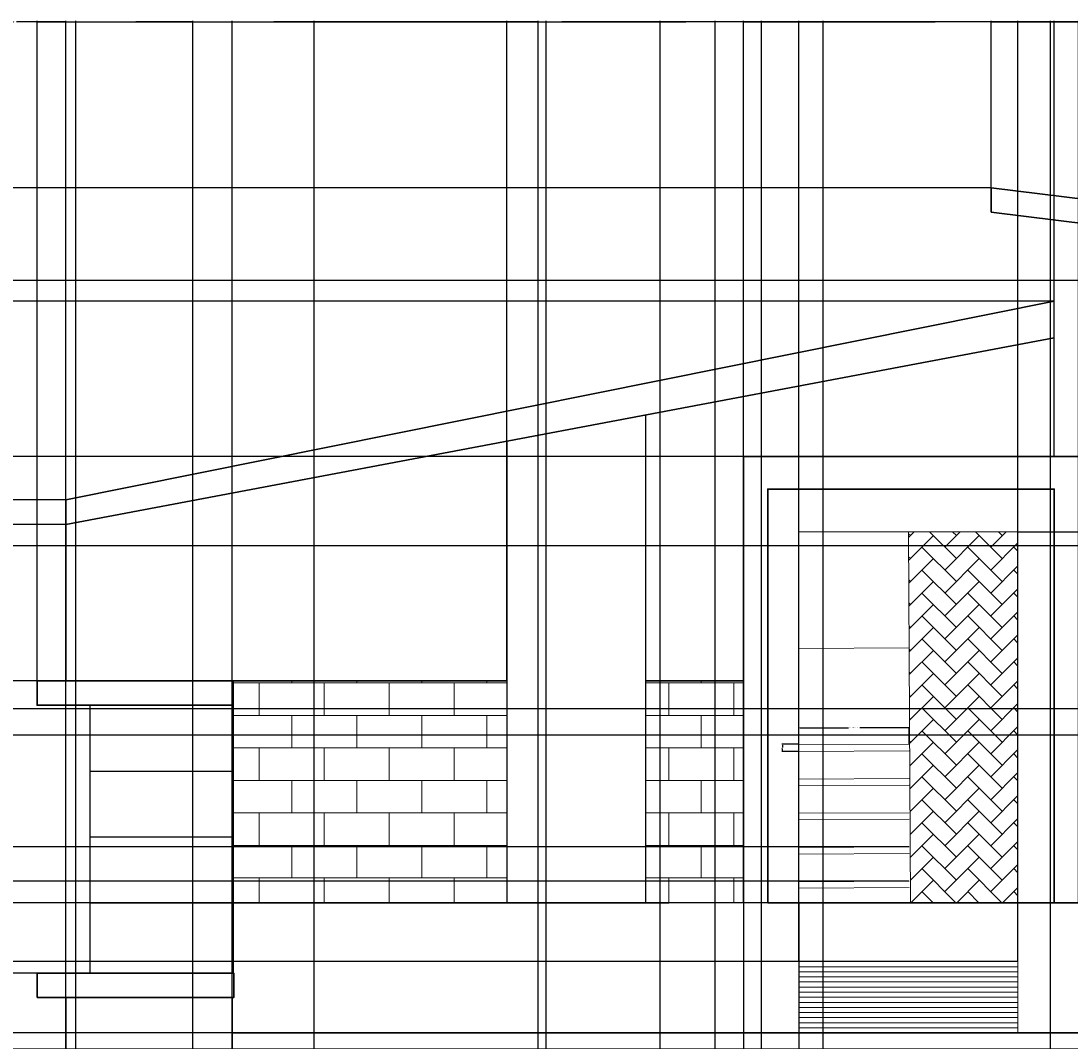
# Model space of a CAD drawing. Units: inches. Extents: x -14 to 886, y 45 to 435.
# Tile 3 of 5: x 125 to 384, y 184 to 435. Entities that reach past the tile are written whole.
import ezdxf

# ---------------------------------------------------------------- set-up
doc = ezdxf.new("R2010")
doc.units = ezdxf.units.IN
doc.header["$MEASUREMENT"] = 0
for name, color, linetype, lineweight in [('A-ANNO-DIMS', 2, 'Continuous', 18), ('A-ELEV-BAND', 7, 'Continuous', 30), ('A-ELEV-PATT', 252, 'Continuous', 13), ('A-ELEV-SCRN', 8, 'Continuous', 18), ('A-ROOF', 7, 'Continuous', 35), ('A-WALL', 7, 'Continuous', 25), ('A-WALL-PATT', 252, 'Continuous', 13), ('L-WALL', 7, 'Continuous', 30)]:
    doc.layers.add(name, color=color, linetype=linetype, lineweight=lineweight)
doc.styles.get("Standard").update_dxf_attribs({"font": 'arial.ttf'})
doc.dimstyles.get("Standard").update_dxf_attribs({"dimtxt": 0.18, "dimasz": 0.18, "dimexe": 0.18, "dimexo": 0.0625, "dimgap": 0.09, "dimtad": 0, "dimtih": 1, "dimtoh": 1, "dimdec": 4, "dimzin": 0, "dimdsep": 46, "dimtxsty": 'Standard', "dimcen": 0.09, "dimadec": 0, "dimazin": 0, "dimtfac": 1, "dimtdec": 4, "dimtofl": 0, "dimtmove": 0, "dimatfit": 3, "dimfxl": 1, "dimtolj": 1, "dimtzin": 0, "dimarcsym": 0})

# ---------------------------------------------------------------- blocks, each defined once
blk = doc.blocks.new('SCREEN-HORIZONTAL-BAR')
for p, q in [((0, 1.61), (27.14, 1.76)), ((0, 0), (27.14, 0.16))]:
    blk.add_line(p, q)
blk = doc.blocks.new('*D6')
at = {"layer": 'A-ANNO-DIMS', "color": 0, "lineweight": -2, "transparency": 16777216}
for p, q in [((316.91, 256.97), (316.91, 261.16)), ((317.09, 260.98), (329.1, 260.98)), ((343.87, 260.98), (331.86, 260.98)), ((344.05, 256.97), (344.05, 261.16))]:
    blk.add_line(p, q, dxfattribs=at)
at = {"layer": 'A-ANNO-DIMS', "color": 0, "transparency": 16777216}
for points in [[(317.09, 261.01), (317.09, 260.95), (316.91, 260.98)], [(343.87, 261.01), (343.87, 260.95), (344.05, 260.98)]]:
    blk.add_solid(points, dxfattribs=at)
at = {"layer": 'Defpoints', "color": 0, "transparency": 16777216}
for p in [(344.05, 260.98), (316.91, 256.91), (344.05, 256.91)]:
    blk.add_point(p, dxfattribs=at)
at = {"layer": 'A-ANNO-DIMS', "color": 0, "transparency": 16777216, "insert": (330.48, 260.98), "char_height": 0.18, "attachment_point": 5}
blk.add_mtext('\\A1;SCREEN BAR 27 TYP.', dxfattribs=at)
blk = doc.blocks.new('*D7')
at = {"layer": 'A-ANNO-DIMS', "color": 0, "lineweight": -2, "transparency": 16777216}
for p, q in [((316.85, 256.91), (312.66, 256.91)), ((312.84, 256.73), (312.84, 256.21)), ((316.85, 255.15), (312.66, 255.15)), ((312.84, 255.33), (312.84, 255.85))]:
    blk.add_line(p, q, dxfattribs=at)
at = {"layer": 'A-ANNO-DIMS', "color": 0, "transparency": 16777216}
for points in [[(312.81, 256.73), (312.87, 256.73), (312.84, 256.91)], [(312.81, 255.33), (312.87, 255.33), (312.84, 255.15)]]:
    blk.add_solid(points, dxfattribs=at)
at = {"layer": 'Defpoints', "color": 0, "transparency": 16777216}
for p in [(312.84, 256.91), (316.91, 256.91), (316.91, 255.15)]:
    blk.add_point(p, dxfattribs=at)
at = {"layer": 'A-ANNO-DIMS', "color": 0, "transparency": 16777216, "insert": (312.84, 256.03), "char_height": 0.18, "attachment_point": 5}
blk.add_mtext('\\A1;2 TYP.', dxfattribs=at)
blk = doc.blocks.new('*D17')
at = {"layer": 'A-ANNO-DIMS', "color": 0, "lineweight": -2, "transparency": 16777216}
for p, q in [((364.17, 393.98), (-13.96, 393.98)), ((-13.78, 393.8), (-13.78, 240.44)), ((-13.78, 86.72), (-13.78, 240.08)), ((111.24, 86.54), (-13.96, 86.54))]:
    blk.add_line(p, q, dxfattribs=at)
at = {"layer": 'A-ANNO-DIMS', "color": 0, "transparency": 16777216}
for points in [[(-13.81, 393.8), (-13.75, 393.8), (-13.78, 393.98)], [(-13.81, 86.72), (-13.75, 86.72), (-13.78, 86.54)]]:
    blk.add_solid(points, dxfattribs=at)
at = {"layer": 'Defpoints', "color": 0, "transparency": 16777216}
for p in [(-13.78, 393.98), (364.23, 393.98), (111.3, 86.54)]:
    blk.add_point(p, dxfattribs=at)
at = {"layer": 'A-ANNO-DIMS', "color": 0, "transparency": 16777216, "insert": (-13.78, 240.26), "char_height": 0.18, "attachment_point": 5}
blk.add_mtext('\\A1;307.44', dxfattribs=at)
blk = doc.blocks.new('*D24')
at = {"layer": 'A-ANNO-DIMS', "color": 0, "lineweight": -2, "transparency": 16777216}
for p, q in [((136.31, 311.03), (-13.96, 311.03)), ((-13.78, 310.85), (-13.78, 198.97)), ((-13.78, 86.72), (-13.78, 198.6)), ((195.24, 86.54), (-13.96, 86.54))]:
    blk.add_line(p, q, dxfattribs=at)
at = {"layer": 'A-ANNO-DIMS', "color": 0, "transparency": 16777216}
for points in [[(-13.81, 310.85), (-13.75, 310.85), (-13.78, 311.03)], [(-13.81, 86.72), (-13.75, 86.72), (-13.78, 86.54)]]:
    blk.add_solid(points, dxfattribs=at)
at = {"layer": 'Defpoints', "color": 0, "transparency": 16777216}
for p in [(-13.78, 311.03), (136.37, 311.03), (195.3, 86.54)]:
    blk.add_point(p, dxfattribs=at)
at = {"layer": 'A-ANNO-DIMS', "color": 0, "transparency": 16777216, "insert": (-13.78, 198.79), "char_height": 0.18, "attachment_point": 5}
blk.add_mtext('\\A1;224.5', dxfattribs=at)
blk = doc.blocks.new('*D25')
at = {"layer": 'A-ANNO-DIMS', "color": 0, "lineweight": -2, "transparency": 16777216}
for p, q in [((136.37, 317.16), (136.37, 435.05)), ((136.55, 434.87), (257.59, 434.87)), ((379.56, 434.87), (258.52, 434.87)), ((379.74, 366.09), (379.74, 435.05))]:
    blk.add_line(p, q, dxfattribs=at)
at = {"layer": 'A-ANNO-DIMS', "color": 0, "transparency": 16777216}
for points in [[(136.55, 434.9), (136.55, 434.84), (136.37, 434.87)], [(379.56, 434.9), (379.56, 434.84), (379.74, 434.87)]]:
    blk.add_solid(points, dxfattribs=at)
at = {"layer": 'Defpoints', "color": 0, "transparency": 16777216}
for p in [(379.74, 434.87), (379.74, 366.03), (136.37, 317.1)]:
    blk.add_point(p, dxfattribs=at)
at = {"layer": 'A-ANNO-DIMS', "color": 0, "transparency": 16777216, "insert": (258.05, 434.87), "char_height": 0.18, "attachment_point": 5}
blk.add_mtext('\\A1;243.36', dxfattribs=at)
blk = doc.blocks.new('*D26')
at = {"layer": 'A-ANNO-DIMS', "color": 0, "lineweight": -2, "transparency": 16777216}
for p, q in [((379.67, 366.03), (-13.96, 366.03)), ((-13.78, 365.85), (-13.78, 341.75)), ((-13.78, 317.28), (-13.78, 341.38)), ((136.31, 317.1), (-13.96, 317.1))]:
    blk.add_line(p, q, dxfattribs=at)
at = {"layer": 'A-ANNO-DIMS', "color": 0, "transparency": 16777216}
for points in [[(-13.81, 365.85), (-13.75, 365.85), (-13.78, 366.03)], [(-13.81, 317.28), (-13.75, 317.28), (-13.78, 317.1)]]:
    blk.add_solid(points, dxfattribs=at)
at = {"layer": 'Defpoints', "color": 0, "transparency": 16777216}
for p in [(-13.78, 366.03), (379.74, 366.03), (136.37, 317.1)]:
    blk.add_point(p, dxfattribs=at)
at = {"layer": 'A-ANNO-DIMS', "color": 0, "transparency": 16777216, "insert": (-13.78, 341.56), "char_height": 0.18, "attachment_point": 5}
blk.add_mtext('\\A1;48.92', dxfattribs=at)
blk = doc.blocks.new('*D27')
at = {"layer": 'A-ANNO-DIMS', "color": 0, "lineweight": -2, "transparency": 16777216}
for p, q in [((136.31, 317.1), (-13.96, 317.1)), ((-13.78, 316.92), (-13.78, 314.25)), ((-13.78, 311.21), (-13.78, 313.89)), ((136.31, 311.03), (-13.96, 311.03))]:
    blk.add_line(p, q, dxfattribs=at)
at = {"layer": 'A-ANNO-DIMS', "color": 0, "transparency": 16777216}
for points in [[(-13.81, 316.92), (-13.75, 316.92), (-13.78, 317.1)], [(-13.81, 311.21), (-13.75, 311.21), (-13.78, 311.03)]]:
    blk.add_solid(points, dxfattribs=at)
at = {"layer": 'Defpoints', "color": 0, "transparency": 16777216}
for p in [(-13.78, 317.1), (136.37, 317.1), (136.37, 311.03)]:
    blk.add_point(p, dxfattribs=at)
at = {"layer": 'A-ANNO-DIMS', "color": 0, "transparency": 16777216, "insert": (-13.78, 314.07), "char_height": 0.18, "attachment_point": 5}
blk.add_mtext('\\A1;6.069', dxfattribs=at)
blk = doc.blocks.new('*D28')
at = {"layer": 'A-ANNO-DIMS', "color": 0, "lineweight": -2, "transparency": 16777216}
for p, q in [((364.23, 394.04), (364.23, 435.05)), ((364.41, 434.87), (456.34, 434.87)), ((549.17, 434.87), (457.25, 434.87)), ((549.35, 371.18), (549.35, 435.05))]:
    blk.add_line(p, q, dxfattribs=at)
at = {"layer": 'A-ANNO-DIMS', "color": 0, "transparency": 16777216}
for points in [[(364.41, 434.9), (364.41, 434.84), (364.23, 434.87)], [(549.17, 434.9), (549.17, 434.84), (549.35, 434.87)]]:
    blk.add_solid(points, dxfattribs=at)
at = {"layer": 'Defpoints', "color": 0, "transparency": 16777216}
for p in [(549.35, 434.87), (364.23, 393.98), (549.35, 371.11)]:
    blk.add_point(p, dxfattribs=at)
at = {"layer": 'A-ANNO-DIMS', "color": 0, "transparency": 16777216, "insert": (456.79, 434.87), "char_height": 0.18, "attachment_point": 5}
blk.add_mtext('\\A1;185.12', dxfattribs=at)
blk = doc.blocks.new('*D29')
at = {"layer": 'A-ANNO-DIMS', "color": 0, "lineweight": -2, "transparency": 16777216}
for p, q in [((364.17, 393.98), (-13.96, 393.98)), ((-13.78, 393.8), (-13.78, 382.73)), ((-13.78, 371.29), (-13.78, 382.37)), ((549.29, 371.11), (-13.96, 371.11))]:
    blk.add_line(p, q, dxfattribs=at)
at = {"layer": 'A-ANNO-DIMS', "color": 0, "transparency": 16777216}
for points in [[(-13.81, 393.8), (-13.75, 393.8), (-13.78, 393.98)], [(-13.81, 371.29), (-13.75, 371.29), (-13.78, 371.11)]]:
    blk.add_solid(points, dxfattribs=at)
at = {"layer": 'Defpoints', "color": 0, "transparency": 16777216}
for p in [(364.23, 393.98), (-13.78, 371.11), (549.35, 371.11)]:
    blk.add_point(p, dxfattribs=at)
at = {"layer": 'A-ANNO-DIMS', "color": 0, "transparency": 16777216, "insert": (-13.78, 382.55), "char_height": 0.18, "attachment_point": 5}
blk.add_mtext('\\A1;22.865', dxfattribs=at)
blk = doc.blocks.new('*D31')
at = {"layer": 'A-ANNO-DIMS', "color": 0, "lineweight": -2, "transparency": 16777216}
for p, q in [((303.24, 327.84), (303.24, 435.05)), ((303.42, 434.87), (344.12, 434.87)), ((385.61, 434.87), (344.91, 434.87)), ((385.79, 327.84), (385.79, 435.05))]:
    blk.add_line(p, q, dxfattribs=at)
at = {"layer": 'A-ANNO-DIMS', "color": 0, "transparency": 16777216}
for points in [[(303.42, 434.9), (303.42, 434.84), (303.24, 434.87)], [(385.61, 434.9), (385.61, 434.84), (385.79, 434.87)]]:
    blk.add_solid(points, dxfattribs=at)
at = {"layer": 'Defpoints', "color": 0, "transparency": 16777216}
for p in [(385.79, 434.87), (303.24, 327.78), (385.79, 327.78)]:
    blk.add_point(p, dxfattribs=at)
at = {"layer": 'A-ANNO-DIMS', "color": 0, "transparency": 16777216, "insert": (344.51, 434.87), "char_height": 0.18, "attachment_point": 5}
blk.add_mtext('\\A1;82.55', dxfattribs=at)
blk = doc.blocks.new('*D32')
at = {"layer": 'A-ANNO-DIMS', "color": 0, "lineweight": -2, "transparency": 16777216}
for p, q in [((303.18, 327.78), (-13.96, 327.78)), ((-13.78, 327.6), (-13.78, 273.01)), ((-13.78, 218.06), (-13.78, 272.65)), ((303.18, 217.88), (-13.96, 217.88))]:
    blk.add_line(p, q, dxfattribs=at)
at = {"layer": 'A-ANNO-DIMS', "color": 0, "transparency": 16777216}
for points in [[(-13.81, 327.6), (-13.75, 327.6), (-13.78, 327.78)], [(-13.81, 218.06), (-13.75, 218.06), (-13.78, 217.88)]]:
    blk.add_solid(points, dxfattribs=at)
at = {"layer": 'Defpoints', "color": 0, "transparency": 16777216}
for p in [(-13.78, 327.78), (303.24, 327.78), (303.24, 217.88)]:
    blk.add_point(p, dxfattribs=at)
at = {"layer": 'A-ANNO-DIMS', "color": 0, "transparency": 16777216, "insert": (-13.78, 272.83), "char_height": 0.18, "attachment_point": 5}
blk.add_mtext('\\A1;109.9', dxfattribs=at)
blk = doc.blocks.new('*D34')
at = {"layer": 'A-ANNO-DIMS', "color": 0, "lineweight": -2, "transparency": 16777216}
for p, q in [((177.3, 179.88), (177.3, 435.05)), ((177.48, 434.87), (285.86, 434.87)), ((395.16, 434.87), (286.79, 434.87)), ((395.34, 179.88), (395.34, 435.05))]:
    blk.add_line(p, q, dxfattribs=at)
at = {"layer": 'A-ANNO-DIMS', "color": 0, "transparency": 16777216}
for points in [[(177.48, 434.9), (177.48, 434.84), (177.3, 434.87)], [(395.16, 434.9), (395.16, 434.84), (395.34, 434.87)]]:
    blk.add_solid(points, dxfattribs=at)
at = {"layer": 'Defpoints', "color": 0, "transparency": 16777216}
for p in [(395.34, 434.87), (177.3, 179.82), (395.34, 179.82)]:
    blk.add_point(p, dxfattribs=at)
at = {"layer": 'A-ANNO-DIMS', "color": 0, "transparency": 16777216, "insert": (286.32, 434.87), "char_height": 0.18, "attachment_point": 5}
blk.add_mtext('\\A1;218.04', dxfattribs=at)
blk = doc.blocks.new('*D35')
at = {"layer": 'A-ANNO-DIMS', "color": 0, "lineweight": -2, "transparency": 16777216}
for p, q in [((395.28, 217.88), (-13.96, 217.88)), ((-13.78, 217.7), (-13.78, 199.03)), ((-13.78, 180), (-13.78, 198.67)), ((395.28, 179.82), (-13.96, 179.82))]:
    blk.add_line(p, q, dxfattribs=at)
at = {"layer": 'A-ANNO-DIMS', "color": 0, "transparency": 16777216}
for points in [[(-13.81, 217.7), (-13.75, 217.7), (-13.78, 217.88)], [(-13.81, 180), (-13.75, 180), (-13.78, 179.82)]]:
    blk.add_solid(points, dxfattribs=at)
at = {"layer": 'Defpoints', "color": 0, "transparency": 16777216}
for p in [(-13.78, 217.88), (395.34, 217.88), (395.34, 179.82)]:
    blk.add_point(p, dxfattribs=at)
at = {"layer": 'A-ANNO-DIMS', "color": 0, "transparency": 16777216, "insert": (-13.78, 198.85), "char_height": 0.18, "attachment_point": 5}
blk.add_mtext('\\A1;38.06', dxfattribs=at)
blk = doc.blocks.new('*D41')
at = {"layer": 'A-ANNO-DIMS', "color": 0, "lineweight": -2, "transparency": 16777216}
for p, q in [((591.24, 259.14), (-13.96, 259.14)), ((-13.78, 258.96), (-13.78, 203.02)), ((-13.78, 146.72), (-13.78, 202.66)), ((537.19, 146.54), (-13.96, 146.54))]:
    blk.add_line(p, q, dxfattribs=at)
at = {"layer": 'A-ANNO-DIMS', "color": 0, "transparency": 16777216}
for points in [[(-13.81, 258.96), (-13.75, 258.96), (-13.78, 259.14)], [(-13.81, 146.72), (-13.75, 146.72), (-13.78, 146.54)]]:
    blk.add_solid(points, dxfattribs=at)
at = {"layer": 'Defpoints', "color": 0, "transparency": 16777216}
for p in [(-13.78, 259.14), (591.3, 259.14), (537.25, 146.54)]:
    blk.add_point(p, dxfattribs=at)
at = {"layer": 'A-ANNO-DIMS', "color": 0, "transparency": 16777216, "insert": (-13.78, 202.84), "char_height": 0.18, "attachment_point": 5}
blk.add_mtext('\\A1;112.6', dxfattribs=at)
blk = doc.blocks.new('*D42')
at = {"layer": 'A-ANNO-DIMS', "color": 0, "lineweight": -2, "transparency": 16777216}
for p, q in [((129.24, 272.54), (-13.96, 272.54)), ((-13.78, 272.36), (-13.78, 236.72)), ((-13.78, 200.72), (-13.78, 236.36)), ((129.24, 200.54), (-13.96, 200.54))]:
    blk.add_line(p, q, dxfattribs=at)
at = {"layer": 'A-ANNO-DIMS', "color": 0, "transparency": 16777216}
for points in [[(-13.81, 272.36), (-13.75, 272.36), (-13.78, 272.54)], [(-13.81, 200.72), (-13.75, 200.72), (-13.78, 200.54)]]:
    blk.add_solid(points, dxfattribs=at)
at = {"layer": 'Defpoints', "color": 0, "transparency": 16777216}
for p in [(-13.78, 272.54), (129.3, 272.54), (129.3, 200.54)]:
    blk.add_point(p, dxfattribs=at)
at = {"layer": 'A-ANNO-DIMS', "color": 0, "transparency": 16777216, "insert": (-13.78, 236.54), "char_height": 0.18, "attachment_point": 5}
blk.add_mtext('\\A1;72', dxfattribs=at)
blk = doc.blocks.new('*D43')
at = {"layer": 'A-ANNO-DIMS', "color": 0, "lineweight": -2, "transparency": 16777216}
for p, q in [((129.3, 272.6), (129.3, 435.05)), ((129.48, 434.87), (186.69, 434.87)), ((244.81, 434.87), (187.6, 434.87)), ((244.99, 272.6), (244.99, 435.05))]:
    blk.add_line(p, q, dxfattribs=at)
at = {"layer": 'A-ANNO-DIMS', "color": 0, "transparency": 16777216}
for points in [[(129.48, 434.9), (129.48, 434.84), (129.3, 434.87)], [(244.81, 434.9), (244.81, 434.84), (244.99, 434.87)]]:
    blk.add_solid(points, dxfattribs=at)
at = {"layer": 'Defpoints', "color": 0, "transparency": 16777216}
for p in [(244.99, 434.87), (129.3, 272.54), (244.99, 272.54)]:
    blk.add_point(p, dxfattribs=at)
at = {"layer": 'A-ANNO-DIMS', "color": 0, "transparency": 16777216, "insert": (187.15, 434.87), "char_height": 0.18, "attachment_point": 5}
blk.add_mtext('\\A1;115.69', dxfattribs=at)
blk = doc.blocks.new('*D45')
at = {"layer": 'A-ANNO-DIMS', "color": 0, "lineweight": -2, "transparency": 16777216}
for p, q in [((197.55, 133.22), (197.55, 435.05)), ((197.73, 434.87), (224.73, 434.87)), ((252.49, 434.87), (225.49, 434.87)), ((252.67, 133.22), (252.67, 435.05))]:
    blk.add_line(p, q, dxfattribs=at)
at = {"layer": 'A-ANNO-DIMS', "color": 0, "transparency": 16777216}
for points in [[(197.73, 434.9), (197.73, 434.84), (197.55, 434.87)], [(252.49, 434.9), (252.49, 434.84), (252.67, 434.87)]]:
    blk.add_solid(points, dxfattribs=at)
at = {"layer": 'Defpoints', "color": 0, "transparency": 16777216}
for p in [(252.67, 434.87), (197.55, 133.16), (252.67, 133.16)]:
    blk.add_point(p, dxfattribs=at)
at = {"layer": 'A-ANNO-DIMS', "color": 0, "transparency": 16777216, "insert": (225.11, 434.87), "char_height": 0.18, "attachment_point": 5}
blk.add_mtext('\\A1;55.11', dxfattribs=at)
blk = doc.blocks.new('*D46')
at = {"layer": 'A-ANNO-DIMS', "color": 0, "lineweight": -2, "transparency": 16777216}
for p, q in [((254.67, 133.22), (254.67, 435.05)), ((254.85, 434.87), (280.95, 434.87)), ((307.49, 434.87), (281.39, 434.87)), ((307.67, 133.22), (307.67, 435.05))]:
    blk.add_line(p, q, dxfattribs=at)
at = {"layer": 'A-ANNO-DIMS', "color": 0, "transparency": 16777216}
for points in [[(254.85, 434.9), (254.85, 434.84), (254.67, 434.87)], [(307.49, 434.9), (307.49, 434.84), (307.67, 434.87)]]:
    blk.add_solid(points, dxfattribs=at)
at = {"layer": 'Defpoints', "color": 0, "transparency": 16777216}
for p in [(307.67, 434.87), (254.67, 133.16), (307.67, 133.16)]:
    blk.add_point(p, dxfattribs=at)
at = {"layer": 'A-ANNO-DIMS', "color": 0, "transparency": 16777216, "insert": (281.17, 434.87), "char_height": 0.18, "attachment_point": 5}
blk.add_mtext('\\A1;53', dxfattribs=at)
blk = doc.blocks.new('*D47')
at = {"layer": 'A-ANNO-DIMS', "color": 0, "lineweight": -2, "transparency": 16777216}
for p, q in [((322.89, 133.22), (322.89, 435.05)), ((323.07, 434.87), (350.46, 434.87)), ((378.65, 434.87), (351.25, 434.87)), ((378.83, 133.22), (378.83, 435.05))]:
    blk.add_line(p, q, dxfattribs=at)
at = {"layer": 'A-ANNO-DIMS', "color": 0, "transparency": 16777216}
for points in [[(323.07, 434.9), (323.07, 434.84), (322.89, 434.87)], [(378.65, 434.9), (378.65, 434.84), (378.83, 434.87)]]:
    blk.add_solid(points, dxfattribs=at)
at = {"layer": 'Defpoints', "color": 0, "transparency": 16777216}
for p in [(378.83, 434.87), (322.89, 133.16), (378.83, 133.16)]:
    blk.add_point(p, dxfattribs=at)
at = {"layer": 'A-ANNO-DIMS', "color": 0, "transparency": 16777216, "insert": (350.86, 434.87), "char_height": 0.18, "attachment_point": 5}
blk.add_mtext('\\A1;55.94', dxfattribs=at)
blk = doc.blocks.new('*D48')
at = {"layer": 'A-ANNO-DIMS', "color": 0, "lineweight": -2, "transparency": 16777216}
for p, q in [((316.91, 203.43), (316.91, 435.05)), ((317.09, 434.87), (343.49, 434.87)), ((370.67, 434.87), (344.27, 434.87)), ((370.85, 203.43), (370.85, 435.05))]:
    blk.add_line(p, q, dxfattribs=at)
at = {"layer": 'A-ANNO-DIMS', "color": 0, "transparency": 16777216}
for points in [[(317.09, 434.9), (317.09, 434.84), (316.91, 434.87)], [(370.67, 434.9), (370.67, 434.84), (370.85, 434.87)]]:
    blk.add_solid(points, dxfattribs=at)
at = {"layer": 'Defpoints', "color": 0, "transparency": 16777216}
for p in [(370.85, 434.87), (316.91, 203.37), (370.85, 203.37)]:
    blk.add_point(p, dxfattribs=at)
at = {"layer": 'A-ANNO-DIMS', "color": 0, "transparency": 16777216, "insert": (343.88, 434.87), "char_height": 0.18, "attachment_point": 5}
blk.add_mtext('\\A1;53.94', dxfattribs=at)
blk = doc.blocks.new('*D49')
at = {"layer": 'A-ANNO-DIMS', "color": 0, "lineweight": -2, "transparency": 16777216}
for p, q in [((370.79, 203.37), (-13.96, 203.37)), ((-13.78, 203.19), (-13.78, 194.78)), ((-13.78, 186), (-13.78, 194.41)), ((370.79, 185.82), (-13.96, 185.82))]:
    blk.add_line(p, q, dxfattribs=at)
at = {"layer": 'A-ANNO-DIMS', "color": 0, "transparency": 16777216}
for points in [[(-13.81, 203.19), (-13.75, 203.19), (-13.78, 203.37)], [(-13.81, 186), (-13.75, 186), (-13.78, 185.82)]]:
    blk.add_solid(points, dxfattribs=at)
at = {"layer": 'Defpoints', "color": 0, "transparency": 16777216}
for p in [(-13.78, 203.37), (370.85, 203.37), (370.85, 185.82)]:
    blk.add_point(p, dxfattribs=at)
at = {"layer": 'A-ANNO-DIMS', "color": 0, "transparency": 16777216, "insert": (-13.78, 194.6), "char_height": 0.18, "attachment_point": 5}
blk.add_mtext('\\A1;17.55', dxfattribs=at)
blk = doc.blocks.new('*D50')
at = {"layer": 'A-ANNO-DIMS', "color": 0, "lineweight": -2, "transparency": 16777216}
for p, q in [((316.91, 309.29), (316.91, 435.05)), ((317.09, 434.87), (343.49, 434.87)), ((370.67, 434.87), (344.27, 434.87)), ((370.85, 309.29), (370.85, 435.05))]:
    blk.add_line(p, q, dxfattribs=at)
at = {"layer": 'A-ANNO-DIMS', "color": 0, "transparency": 16777216}
for points in [[(317.09, 434.9), (317.09, 434.84), (316.91, 434.87)], [(370.67, 434.9), (370.67, 434.84), (370.85, 434.87)]]:
    blk.add_solid(points, dxfattribs=at)
at = {"layer": 'Defpoints', "color": 0, "transparency": 16777216}
for p in [(370.85, 434.87), (316.91, 309.22), (370.85, 309.22)]:
    blk.add_point(p, dxfattribs=at)
at = {"layer": 'A-ANNO-DIMS', "color": 0, "transparency": 16777216, "insert": (343.88, 434.87), "char_height": 0.18, "attachment_point": 5}
blk.add_mtext('\\A1;53.94', dxfattribs=at)
blk = doc.blocks.new('*D51')
at = {"layer": 'A-ANNO-DIMS', "color": 0, "lineweight": -2, "transparency": 16777216}
for p, q in [((370.91, 309.22), (885.58, 309.22)), ((885.4, 309.04), (885.4, 263.74)), ((885.4, 218.06), (885.4, 263.37)), ((370.91, 217.88), (885.58, 217.88))]:
    blk.add_line(p, q, dxfattribs=at)
at = {"layer": 'A-ANNO-DIMS', "color": 0, "transparency": 16777216}
for points in [[(885.37, 309.04), (885.43, 309.04), (885.4, 309.22)], [(885.37, 218.06), (885.43, 218.06), (885.4, 217.88)]]:
    blk.add_solid(points, dxfattribs=at)
at = {"layer": 'Defpoints', "color": 0, "transparency": 16777216}
for p in [(370.85, 309.22), (885.4, 309.22), (370.85, 217.88)]:
    blk.add_point(p, dxfattribs=at)
at = {"layer": 'A-ANNO-DIMS', "color": 0, "transparency": 16777216, "insert": (885.4, 263.55), "char_height": 0.18, "attachment_point": 5}
blk.add_mtext('\\A1;91.34', dxfattribs=at)
blk = doc.blocks.new('*D53')
at = {"layer": 'A-ANNO-DIMS', "color": 0, "lineweight": -2, "transparency": 16777216}
for p, q in [((444.97, 305.77), (-13.96, 305.77)), ((-13.78, 305.59), (-13.78, 285.9)), ((-13.78, 265.85), (-13.78, 285.54)), ((444.97, 265.67), (-13.96, 265.67))]:
    blk.add_line(p, q, dxfattribs=at)
at = {"layer": 'A-ANNO-DIMS', "color": 0, "transparency": 16777216}
for points in [[(-13.81, 305.59), (-13.75, 305.59), (-13.78, 305.77)], [(-13.81, 265.85), (-13.75, 265.85), (-13.78, 265.67)]]:
    blk.add_solid(points, dxfattribs=at)
at = {"layer": 'Defpoints', "color": 0, "transparency": 16777216}
for p in [(-13.78, 305.77), (445.04, 305.77), (445.04, 265.67)]:
    blk.add_point(p, dxfattribs=at)
at = {"layer": 'A-ANNO-DIMS', "color": 0, "transparency": 16777216, "insert": (-13.78, 285.72), "char_height": 0.18, "attachment_point": 5}
blk.add_mtext('\\A1;40.104', dxfattribs=at)
blk = doc.blocks.new('*D55')
at = {"layer": 'A-ANNO-DIMS', "color": 0, "lineweight": -2, "transparency": 16777216}
for p, q in [((444.97, 265.67), (-13.96, 265.67)), ((-13.78, 265.49), (-13.78, 223.93)), ((-13.78, 182.01), (-13.78, 223.57)), ((444.97, 181.83), (-13.96, 181.83))]:
    blk.add_line(p, q, dxfattribs=at)
at = {"layer": 'A-ANNO-DIMS', "color": 0, "transparency": 16777216}
for points in [[(-13.81, 265.49), (-13.75, 265.49), (-13.78, 265.67)], [(-13.81, 182.01), (-13.75, 182.01), (-13.78, 181.83)]]:
    blk.add_solid(points, dxfattribs=at)
at = {"layer": 'Defpoints', "color": 0, "transparency": 16777216}
for p in [(-13.78, 265.67), (445.04, 265.67), (445.04, 181.83)]:
    blk.add_point(p, dxfattribs=at)
at = {"layer": 'A-ANNO-DIMS', "color": 0, "transparency": 16777216, "insert": (-13.78, 223.75), "char_height": 0.18, "attachment_point": 5}
blk.add_mtext('\\A1;83.84', dxfattribs=at)
blk = doc.blocks.new('*D60')
at = {"layer": 'A-ANNO-DIMS', "color": 0, "lineweight": -2, "transparency": 16777216}
for p, q in [((343.98, 231.64), (-13.96, 231.64)), ((-13.78, 231.46), (-13.78, 227.61)), ((-13.78, 223.39), (-13.78, 227.25)), ((343.98, 223.21), (-13.96, 223.21))]:
    blk.add_line(p, q, dxfattribs=at)
at = {"layer": 'A-ANNO-DIMS', "color": 0, "transparency": 16777216}
for points in [[(-13.81, 231.46), (-13.75, 231.46), (-13.78, 231.64)], [(-13.81, 223.39), (-13.75, 223.39), (-13.78, 223.21)]]:
    blk.add_solid(points, dxfattribs=at)
at = {"layer": 'Defpoints', "color": 0, "transparency": 16777216}
for p in [(-13.78, 231.64), (344.05, 231.64), (344.05, 223.21)]:
    blk.add_point(p, dxfattribs=at)
at = {"layer": 'A-ANNO-DIMS', "color": 0, "transparency": 16777216, "insert": (-13.78, 227.43), "char_height": 0.18, "attachment_point": 5}
blk.add_mtext('\\A1;8.424', dxfattribs=at)
blk = doc.blocks.new('*D61')
at = {"layer": 'A-ANNO-DIMS', "color": 0, "lineweight": -2, "transparency": 16777216}
for p, q in [((282.73, 173.88), (282.73, 435.05)), ((282.91, 434.87), (289.04, 434.87)), ((296.09, 434.87), (289.96, 434.87)), ((296.27, 173.88), (296.27, 435.05))]:
    blk.add_line(p, q, dxfattribs=at)
at = {"layer": 'A-ANNO-DIMS', "color": 0, "transparency": 16777216}
for points in [[(282.91, 434.9), (282.91, 434.84), (282.73, 434.87)], [(296.09, 434.9), (296.09, 434.84), (296.27, 434.87)]]:
    blk.add_solid(points, dxfattribs=at)
at = {"layer": 'Defpoints', "color": 0, "transparency": 16777216}
for p in [(296.27, 434.87), (282.73, 173.82), (296.27, 173.82)]:
    blk.add_point(p, dxfattribs=at)
at = {"layer": 'A-ANNO-DIMS', "color": 0, "transparency": 16777216, "insert": (289.5, 434.87), "char_height": 0.18, "attachment_point": 5}
blk.add_mtext('\\A1;13.538', dxfattribs=at)
blk = doc.blocks.new('*D63')
at = {"layer": 'A-ANNO-DIMS', "color": 0, "lineweight": -2, "transparency": 16777216}
for p, q in [((138.83, 133.13), (138.83, 435.05)), ((139.01, 434.87), (152.85, 434.87)), ((167.48, 434.87), (153.64, 434.87)), ((167.66, 133.13), (167.66, 435.05))]:
    blk.add_line(p, q, dxfattribs=at)
at = {"layer": 'A-ANNO-DIMS', "color": 0, "transparency": 16777216}
for points in [[(139.01, 434.9), (139.01, 434.84), (138.83, 434.87)], [(167.48, 434.9), (167.48, 434.84), (167.66, 434.87)]]:
    blk.add_solid(points, dxfattribs=at)
at = {"layer": 'Defpoints', "color": 0, "transparency": 16777216}
for p in [(167.66, 434.87), (138.83, 133.07), (167.66, 133.07)]:
    blk.add_point(p, dxfattribs=at)
at = {"layer": 'A-ANNO-DIMS', "color": 0, "transparency": 16777216, "insert": (153.25, 434.87), "char_height": 0.18, "attachment_point": 5}
blk.add_mtext('\\A1;28.83', dxfattribs=at)
blk = doc.blocks.new('*D65')
at = {"layer": 'A-ANNO-DIMS', "color": 0, "lineweight": -2, "transparency": 16777216}
for p, q in [((111.3, 158.6), (111.3, 435.05)), ((111.48, 434.87), (123.44, 434.87)), ((136.19, 434.87), (124.23, 434.87)), ((136.37, 158.6), (136.37, 435.05))]:
    blk.add_line(p, q, dxfattribs=at)
at = {"layer": 'A-ANNO-DIMS', "color": 0, "transparency": 16777216}
for points in [[(111.48, 434.9), (111.48, 434.84), (111.3, 434.87)], [(136.19, 434.9), (136.19, 434.84), (136.37, 434.87)]]:
    blk.add_solid(points, dxfattribs=at)
at = {"layer": 'Defpoints', "color": 0, "transparency": 16777216}
for p in [(136.37, 434.87), (111.3, 158.54), (136.37, 158.54)]:
    blk.add_point(p, dxfattribs=at)
at = {"layer": 'A-ANNO-DIMS', "color": 0, "transparency": 16777216, "insert": (123.84, 434.87), "char_height": 0.18, "attachment_point": 5}
blk.add_mtext('\\A1;25.07', dxfattribs=at)
blk = doc.blocks.new('*D66')
at = {"layer": 'A-ANNO-DIMS', "color": 0, "lineweight": -2, "transparency": 16777216}
for p, q in [((303.24, 217.82), (303.24, 45.47)), ((316.91, 217.82), (316.91, 45.47)), ((303.42, 45.65), (309.69, 45.65)), ((316.73, 45.65), (310.46, 45.65))]:
    blk.add_line(p, q, dxfattribs=at)
at = {"layer": 'A-ANNO-DIMS', "color": 0, "transparency": 16777216}
for points in [[(303.42, 45.68), (303.42, 45.62), (303.24, 45.65)], [(316.73, 45.68), (316.73, 45.62), (316.91, 45.65)]]:
    blk.add_solid(points, dxfattribs=at)
at = {"layer": 'Defpoints', "color": 0, "transparency": 16777216}
for p in [(303.24, 217.88), (316.91, 217.88), (316.91, 45.65)]:
    blk.add_point(p, dxfattribs=at)
at = {"layer": 'A-ANNO-DIMS', "color": 0, "transparency": 16777216, "insert": (310.07, 45.65), "char_height": 0.18, "attachment_point": 5}
blk.add_mtext('\\A1;13.67', dxfattribs=at)

msp = doc.modelspace()

# ---------------------------------------------------------------- hatches: boundary and pattern name
at = {"layer": 'A-ELEV-PATT'}
h = msp.add_hatch(dxfattribs=at)
h.set_pattern_fill('LINE', color=256, scale=10.04365, style=0)
h.paths.add_polyline_path([(370.8507, 185.8201), (316.9091, 185.8201), (316.9091, 203.3712), (370.8507, 203.3712)])
at = {"layer": 'A-WALL-PATT'}
h = msp.add_hatch(dxfattribs=at)
h.set_pattern_fill('AR-HBONE', color=256)
h.set_pattern_definition([(45, (-43.1423, 0), (0, 5.656854), [12, -4]), (135, (-40.314, 2.8284), (4e-16, 5.656854), [12, -4])])
h.paths.add_polyline_path([(370.8507, 309.2241), (343.8799, 309.2241), (344.4075, 217.8839), (370.8507, 217.8839)])
h = msp.add_hatch(dxfattribs=at)
h.set_pattern_fill('AR-B816', color=256)
h.paths.add_polyline_path([(244.9899, 272.5389), (177.5892, 272.5389), (177.5892, 217.8839), (244.9899, 217.8839)])
h = msp.add_hatch(dxfattribs=at)
h.set_pattern_fill('AR-B816', color=256)
h.set_pattern_definition([(0, (-43.142, 0), (0, 8), []), (90, (-43.142, 0), (-8, 8), [8, -8])])
h.paths.add_polyline_path([(303.2386, 272.5389), (279.2386, 272.5389), (279.2386, 217.8839), (303.2386, 217.8839)])

# ---------------------------------------------------------------- linework, layer by layer
at = {"layer": 'A-ELEV-BAND'}
for p, q in [((303.2386, 272.5389), (279.2386, 272.5389)), ((142.3714, 217.8839), (284.8577, 217.8839)), ((177.7241, 194.5389), (129.3024, 194.5389)), ((231.2386, 185.8201), (279.2386, 185.8201))]:
    msp.add_line(p, q, dxfattribs=at)
for points in [[(303.2386, 327.7815), (303.2386, 217.8839), (303.2386, 327.7815), (385.7908, 327.7815), (385.7908, 217.8839)], [(379.7908, 217.8839), (379.7908, 319.7815), (309.2386, 319.7815), (309.2386, 217.8839), (395.3394, 217.8839), (395.3394, 179.8201), (177.3024, 179.8201)], [(244.9899, 272.5389), (129.3024, 272.5389), (129.3024, 266.5389), (177.5892, 266.5389)], [(177.3024, 185.8201), (395.3394, 185.8201), (537.2506, 185.8201)]]:
    msp.add_lwpolyline(points, dxfattribs=at)
msp.add_lwpolyline([(129.3024, 194.5389), (177.7241, 194.5389), (177.7241, 200.5389), (129.3024, 200.5389)], close=True, dxfattribs=at)
at = {"layer": 'A-ELEV-SCRN'}
for p, q in [((343.8799, 309.2241), (344.4075, 217.8839)), ((316.9091, 280.4819), (344.045, 280.6387))]:
    msp.add_line(p, q, dxfattribs=at)
msp.add_lwpolyline([(370.8507, 217.8839), (370.8507, 309.2241), (316.9091, 309.2241), (316.9091, 217.8839)], dxfattribs=at)
msp.add_lwpolyline([(370.8507, 185.8201), (316.9091, 185.8201), (316.9091, 203.3712), (370.8507, 203.3712)], close=True, dxfattribs=at)
at = {"layer": 'A-ROOF'}
msp.add_line((136.3714, 311.0336), (379.7355, 356.9881), dxfattribs=at)
msp.add_lwpolyline([(364.2304, 387.9341), (364.2304, 393.9797), (549.3534, 371.1143), (549.3534, 365.0687)], close=True, dxfattribs=at)
msp.add_lwpolyline([(136.3714, 272.5389), (136.3714, 317.1024), (379.7355, 366.0265)], dxfattribs=at)
at = {"layer": 'A-WALL'}
for p, q in [((379.7355, 327.7815), (379.7355, 386.019)), ((244.9899, 331.544), (244.9899, 217.8839)), ((177.5892, 272.5389), (177.5892, 200.5389)), ((136.3714, 200.5389), (136.3714, 266.5389)), ((142.3714, 200.5389), (142.3714, 266.5389)), ((142.3714, 250.3206), (177.7241, 250.3206)), ((142.3714, 234.1022), (177.7241, 234.1022))]:
    msp.add_line(p, q, dxfattribs=at)
for points in [[(309.2386, 217.8839), (279.2386, 217.8839), (279.2386, 338.0112)], [(136.3714, 194.5389), (136.3714, 158.5389), (195.3024, 158.5389)]]:
    msp.add_lwpolyline(points, dxfattribs=at)
at = {"layer": 'L-WALL'}
msp.add_line((177.3024, 86.5389), (177.3024, 194.5389), dxfattribs=at)

# ---------------------------------------------------------------- block references
at = {"layer": 'A-ELEV-SCRN'}
msp.add_blockref('SCREEN-HORIZONTAL-BAR', (316.9091, 255.1471), dxfattribs=at)
at = {"layer": 'A-ELEV-SCRN', "rotation": 180}
for p in [(344.045, 248.4875), (344.045, 240.0633), (344.045, 231.6392), (344.045, 223.215)]:
    msp.add_blockref('SCREEN-HORIZONTAL-BAR', p, dxfattribs=at)

# ---------------------------------------------------------------- dimensions: what is measured, and where the dimension line sits
at = {"layer": 'A-ANNO-DIMS'}
for base, p1, p2, override, picture, middle in [((136.3714, 434.8697), (111.3024, 158.5389), (136.3714, 158.5389), {"dimdec": 2, "dimlfac": 1, "dimrnd": 0, "dimzin": 0, "dimdsep": 46, "dimlunit": 2}, '*D65', (123.8369, 434.8697)), ((244.9899, 434.8697), (129.3024, 272.5389), (244.9899, 272.5389), {"dimdec": 2, "dimlfac": 1, "dimrnd": 0, "dimzin": 0, "dimdsep": 46, "dimlunit": 2}, '*D43', (187.1461, 434.8697)), ((379.7355, 434.8697), (136.3714, 317.1024), (379.7355, 366.0265), {"dimdec": 2, "dimlfac": 1, "dimrnd": 0, "dimzin": 0, "dimdsep": 46, "dimlunit": 2}, '*D25', (258.0535, 434.8697)), ((167.6621, 434.8697), (138.8348, 133.0686), (167.6621, 133.0686), {"dimdec": 2, "dimlfac": 1, "dimrnd": 0, "dimzin": 0, "dimdsep": 46, "dimlunit": 2}, '*D63', (153.2485, 434.8697)), ((395.3394, 434.8697), (177.3024, 179.8201), (395.3394, 179.8201), {"dimdec": 2, "dimlfac": 1, "dimrnd": 0, "dimzin": 0, "dimdsep": 46, "dimlunit": 2}, '*D34', (286.3209, 434.8697)), ((252.6671, 434.8697), (197.5542, 133.1624), (252.6671, 133.1624), {"dimdec": 2, "dimlfac": 1, "dimrnd": 0, "dimzin": 0, "dimdsep": 46, "dimlunit": 2}, '*D45', (225.1107, 434.8697)), ((307.6671, 434.8697), (254.6671, 133.1624), (307.6671, 133.1624), {"dimdec": 0, "dimlfac": 1, "dimrnd": 0, "dimzin": 0, "dimdsep": 46, "dimlunit": 2}, '*D46', (281.1671, 434.8697)), ((296.2693, 434.8697), (282.7312, 173.8201), (296.2693, 173.8201), {"dimdec": 3, "dimlfac": 1, "dimrnd": 0, "dimzin": 0, "dimdsep": 46, "dimlunit": 2}, '*D61', (289.5003, 434.8697)), ((385.7908, 434.8697), (303.2386, 327.7815), (385.7908, 327.7815), {"dimdec": 2, "dimlfac": 1, "dimrnd": 0, "dimzin": 0, "dimdsep": 46, "dimlunit": 2}, '*D31', (344.5147, 434.8697)), ((370.8507, 434.8697), (316.9091, 203.3712), (370.8507, 203.3712), {"dimdec": 2, "dimlfac": 1, "dimrnd": 0, "dimzin": 0, "dimdsep": 46, "dimlunit": 2}, '*D48', (343.8799, 434.8697)), ((370.8507, 434.8697), (316.9091, 309.2241), (370.8507, 309.2241), {"dimdec": 2, "dimlfac": 1, "dimrnd": 0, "dimzin": 0, "dimdsep": 46, "dimlunit": 2}, '*D50', (343.8799, 434.8697)), ((378.8292, 434.8697), (322.8853, 133.1624), (378.8292, 133.1624), {"dimdec": 2, "dimlfac": 1, "dimrnd": 0, "dimzin": 0, "dimdsep": 46, "dimlunit": 2}, '*D47', (350.8573, 434.8697)), ((549.3534, 434.8697), (364.2304, 393.9797), (549.3534, 371.1143), {"dimdec": 2, "dimlfac": 1, "dimrnd": 0, "dimzin": 0, "dimdsep": 46, "dimlunit": 2}, '*D28', (456.7919, 434.8697)), ((316.9091, 45.6489), (303.2386, 217.8839), (316.9091, 217.8839), {"dimdec": 2, "dimlfac": 1, "dimrnd": 0, "dimzin": 0, "dimdsep": 46, "dimlunit": 2}, '*D66', (310.0739, 45.6489))]:
    dim = msp.add_linear_dim(base=base, p1=p1, p2=p2, dimstyle='Standard', override=override, dxfattribs=at)
    dim.commit()
    dim.dimension.update_dxf_attribs({"geometry": picture, "text_midpoint": middle})
for base, p1, p2, override, picture, middle in [((-13.7769, 393.9797), (111.3024, 86.5389), (364.2304, 393.9797), {"dimdec": 2, "dimlfac": 1, "dimrnd": 0, "dimzin": 0, "dimdsep": 46, "dimlunit": 2}, '*D17', (-13.7769, 240.2593)), ((-13.7769, 371.1143), (364.2304, 393.9797), (549.3534, 371.1143), {"dimdec": 3, "dimlfac": 1, "dimrnd": 0, "dimzin": 0, "dimdsep": 46, "dimlunit": 2}, '*D29', (-13.7769, 382.547)), ((-13.7769, 366.0265), (136.3714, 317.1024), (379.7355, 366.0265), {"dimdec": 2, "dimlfac": 1, "dimrnd": 0, "dimzin": 0, "dimdsep": 46, "dimlunit": 2}, '*D26', (-13.7769, 341.5645)), ((-13.7769, 327.7815), (303.2386, 217.8839), (303.2386, 327.7815), {"dimdec": 1, "dimlfac": 1, "dimrnd": 0, "dimzin": 0, "dimdsep": 46, "dimlunit": 2}, '*D32', (-13.7769, 272.8327)), ((-13.7769, 317.1024), (136.3714, 311.0336), (136.3714, 317.1024), {"dimdec": 3, "dimlfac": 1, "dimrnd": 0, "dimzin": 0, "dimdsep": 46, "dimlunit": 2}, '*D27', (-13.7769, 314.068)), ((-13.7769, 311.0336), (195.3024, 86.5389), (136.3714, 311.0336), {"dimdec": 1, "dimlfac": 1, "dimrnd": 0, "dimzin": 0, "dimdsep": 46, "dimlunit": 2}, '*D24', (-13.7769, 198.7862)), ((885.401, 309.2241), (370.8507, 217.8839), (370.8507, 309.2241), {"dimdec": 2, "dimlfac": 1, "dimrnd": 0, "dimzin": 0, "dimdsep": 46, "dimlunit": 2}, '*D51', (885.401, 263.554)), ((-13.7769, 305.7727), (445.0372, 265.6686), (445.0372, 305.7727), {"dimdec": 3, "dimlfac": 1, "dimrnd": 0, "dimzin": 0, "dimdsep": 46, "dimlunit": 2}, '*D53', (-13.7769, 285.7207)), ((-13.7769, 272.5389), (129.3024, 200.5389), (129.3024, 272.5389), {"dimdec": 0, "dimlfac": 1, "dimrnd": 0, "dimzin": 0, "dimdsep": 46, "dimlunit": 2}, '*D42', (-13.7769, 236.5389)), ((-13.7769, 265.6686), (445.0372, 181.8319), (445.0372, 265.6686), {"dimdec": 2, "dimlfac": 1, "dimrnd": 0, "dimzin": 0, "dimdsep": 46, "dimlunit": 2}, '*D55', (-13.7769, 223.7503)), ((-13.7769, 259.1435), (537.2506, 146.5389), (591.3024, 259.1435), {"dimdec": 1, "dimlfac": 1, "dimrnd": 0, "dimzin": 0, "dimdsep": 46, "dimlunit": 2}, '*D41', (-13.7769, 202.8412)), ((-13.7769, 231.6392), (344.045, 223.215), (344.045, 231.6392), {"dimdec": 3, "dimlfac": 1, "dimrnd": 0, "dimzin": 0, "dimdsep": 46, "dimlunit": 2}, '*D60', (-13.7769, 227.4271)), ((-13.7769, 217.8839), (395.3394, 179.8201), (395.3394, 217.8839), {"dimdec": 2, "dimlfac": 1, "dimrnd": 0, "dimzin": 0, "dimdsep": 46, "dimlunit": 2}, '*D35', (-13.7769, 198.852)), ((-13.7769, 203.3712), (370.8507, 185.8201), (370.8507, 203.3712), {"dimdec": 2, "dimlfac": 1, "dimrnd": 0, "dimzin": 0, "dimdsep": 46, "dimlunit": 2}, '*D49', (-13.7769, 194.5957))]:
    dim = msp.add_linear_dim(base=base, p1=p1, p2=p2, angle=90, dimstyle='Standard', override=override, dxfattribs=at)
    dim.commit()
    dim.dimension.update_dxf_attribs({"geometry": picture, "text_midpoint": middle})
dim = msp.add_linear_dim(base=(344.045, 260.9821), p1=(316.9091, 256.9117), p2=(344.045, 256.9117), text='SCREEN BAR <> TYP.', dimstyle='Standard', override={"dimdec": 0, "dimlfac": 1, "dimrnd": 0, "dimzin": 0, "dimdsep": 46, "dimlunit": 2}, dxfattribs=at)
dim.commit()
dim.dimension.update_dxf_attribs({"geometry": '*D6', "text_midpoint": (330.4771, 260.9821)})
dim = msp.add_linear_dim(base=(312.8387, 256.9117), p1=(316.9091, 255.1471), p2=(316.9091, 256.9117), angle=90, text='<> TYP.', dimstyle='Standard', override={"dimdec": 0, "dimlfac": 1, "dimrnd": 0, "dimzin": 0, "dimdsep": 46, "dimlunit": 2}, dxfattribs=at)
dim.commit()
dim.dimension.update_dxf_attribs({"geometry": '*D7', "text_midpoint": (312.8387, 256.0294)})

doc.saveas('drawing.dxf')
